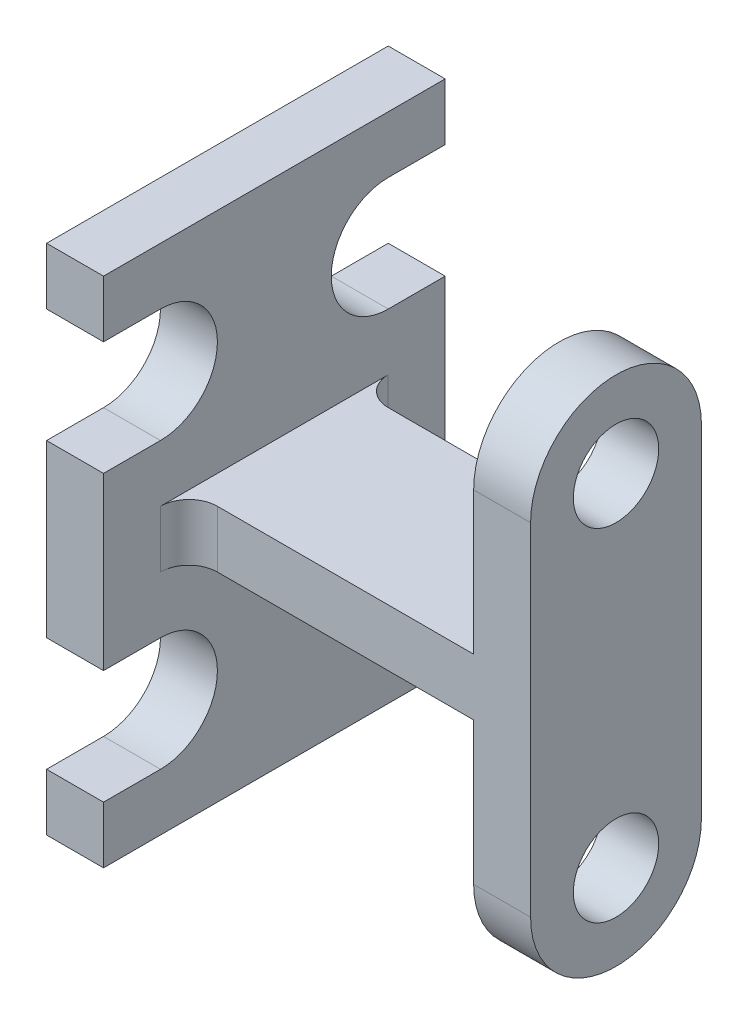
ISO-10303-21;
HEADER;
FILE_DESCRIPTION(('STEP AP214'),'2;1');
FILE_NAME('part.step','',(''),(''),'','','');
FILE_SCHEMA(('AUTOMOTIVE_DESIGN { 1 0 10303 214 1 1 1 1 }'));
ENDSEC;
DATA;
#1=APPLICATION_CONTEXT('core data for automotive mechanical design processes');
#2=APPLICATION_PROTOCOL_DEFINITION('international standard','automotive_design',2000,#1);
#3=PRODUCT_CONTEXT('',#1,'mechanical');
#4=PRODUCT('Part','Part','',(#3));
#5=PRODUCT_RELATED_PRODUCT_CATEGORY('part','',(#4));
#6=PRODUCT_DEFINITION_FORMATION('','',#4);
#7=PRODUCT_DEFINITION_CONTEXT('part definition',#1,'design');
#8=PRODUCT_DEFINITION('design','',#6,#7);
#9=PRODUCT_DEFINITION_SHAPE('','',#8);
#10=(LENGTH_UNIT() NAMED_UNIT(*) SI_UNIT(.MILLI.,.METRE.));
#11=(NAMED_UNIT(*) PLANE_ANGLE_UNIT() SI_UNIT($,.RADIAN.));
#12=(NAMED_UNIT(*) SI_UNIT($,.STERADIAN.) SOLID_ANGLE_UNIT());
#13=UNCERTAINTY_MEASURE_WITH_UNIT(LENGTH_MEASURE(1.E-05),#10,'distance_accuracy_value','');
#14=(GEOMETRIC_REPRESENTATION_CONTEXT(3) GLOBAL_UNCERTAINTY_ASSIGNED_CONTEXT((#13)) GLOBAL_UNIT_ASSIGNED_CONTEXT((#10,
#11,#12)) REPRESENTATION_CONTEXT('',''));
#15=CARTESIAN_POINT('',(0.,0.,0.));
#16=DIRECTION('',(0.,0.,1.));
#17=DIRECTION('',(1.,0.,0.));
#18=AXIS2_PLACEMENT_3D('',#15,#16,#17);
#19=CARTESIAN_POINT('',(10.,4.99999999999997,60.));
#20=DIRECTION('',(-1.,0.,0.));
#21=DIRECTION('',(0.,0.,1.));
#22=AXIS2_PLACEMENT_3D('',#19,#20,#21);
#23=PLANE('',#22);
#24=DIRECTION('',(0.,0.,-1.));
#25=VECTOR('',#24,1.);
#26=CARTESIAN_POINT('',(10.,4.99999999999997,60.));
#27=LINE('',#26,#25);
#28=CARTESIAN_POINT('',(10.,4.99999999999997,50.));
#29=VERTEX_POINT('',#28);
#30=CARTESIAN_POINT('',(10.,4.99999999999997,10.));
#31=VERTEX_POINT('',#30);
#32=EDGE_CURVE('E418',#29,#31,#27,.T.);
#33=ORIENTED_EDGE('',*,*,#32,.T.);
#34=DIRECTION('',(0.,1.,0.));
#35=VECTOR('',#34,1.);
#36=CARTESIAN_POINT('',(10.,-5.00000000000006,10.));
#37=LINE('',#36,#35);
#38=CARTESIAN_POINT('',(10.,-5.00000000000006,10.));
#39=VERTEX_POINT('',#38);
#40=EDGE_CURVE('E432',#31,#39,#37,.F.);
#41=ORIENTED_EDGE('',*,*,#40,.T.);
#42=DIRECTION('',(0.,0.,-1.));
#43=VECTOR('',#42,1.);
#44=CARTESIAN_POINT('',(10.,-5.00000000000006,60.));
#45=LINE('',#44,#43);
#46=CARTESIAN_POINT('',(10.,-5.00000000000006,50.));
#47=VERTEX_POINT('',#46);
#48=EDGE_CURVE('E423',#47,#39,#45,.T.);
#49=ORIENTED_EDGE('',*,*,#48,.F.);
#50=DIRECTION('',(0.,1.,0.));
#51=VECTOR('',#50,1.);
#52=CARTESIAN_POINT('',(10.,4.99999999999997,50.));
#53=LINE('',#52,#51);
#54=EDGE_CURVE('E431',#47,#29,#53,.T.);
#55=ORIENTED_EDGE('',*,*,#54,.T.);
#56=EDGE_LOOP('',(#33,#41,#49,#55));
#57=FACE_BOUND('',#56,.T.);
#58=DIRECTION('',(0.,1.,0.));
#59=VECTOR('',#58,1.);
#60=CARTESIAN_POINT('',(10.,4.99999999999997,60.));
#61=LINE('',#60,#59);
#62=CARTESIAN_POINT('',(10.,35.,60.));
#63=VERTEX_POINT('',#62);
#64=CARTESIAN_POINT('',(10.,45.,60.));
#65=VERTEX_POINT('',#64);
#66=EDGE_CURVE('E387',#63,#65,#61,.T.);
#67=ORIENTED_EDGE('',*,*,#66,.F.);
#68=DIRECTION('',(0.,0.,-1.));
#69=VECTOR('',#68,1.);
#70=CARTESIAN_POINT('',(10.,35.,0.));
#71=LINE('',#70,#69);
#72=CARTESIAN_POINT('',(10.,35.,50.));
#73=VERTEX_POINT('',#72);
#74=EDGE_CURVE('E311',#63,#73,#71,.T.);
#75=ORIENTED_EDGE('',*,*,#74,.T.);
#76=CARTESIAN_POINT('',(10.,25.,50.));
#77=DIRECTION('',(-1.,0.,0.));
#78=DIRECTION('',(0.,0.,1.));
#79=AXIS2_PLACEMENT_3D('',#76,#77,#78);
#80=CIRCLE('',#79,10.);
#81=CARTESIAN_POINT('',(10.,15.,50.));
#82=VERTEX_POINT('',#81);
#83=EDGE_CURVE('E304',#82,#73,#80,.F.);
#84=ORIENTED_EDGE('',*,*,#83,.F.);
#85=DIRECTION('',(0.,0.,1.));
#86=VECTOR('',#85,1.);
#87=CARTESIAN_POINT('',(10.,15.,0.));
#88=LINE('',#87,#86);
#89=CARTESIAN_POINT('',(10.,15.,60.));
#90=VERTEX_POINT('',#89);
#91=EDGE_CURVE('E310',#82,#90,#88,.T.);
#92=ORIENTED_EDGE('',*,*,#91,.T.);
#93=CARTESIAN_POINT('',(10.,-15.,60.));
#94=VERTEX_POINT('',#93);
#95=EDGE_CURVE('E394',#94,#90,#61,.T.);
#96=ORIENTED_EDGE('',*,*,#95,.F.);
#97=DIRECTION('',(0.,0.,-1.));
#98=VECTOR('',#97,1.);
#99=CARTESIAN_POINT('',(10.,-15.,0.));
#100=LINE('',#99,#98);
#101=CARTESIAN_POINT('',(10.,-15.,50.));
#102=VERTEX_POINT('',#101);
#103=EDGE_CURVE('E277',#94,#102,#100,.T.);
#104=ORIENTED_EDGE('',*,*,#103,.T.);
#105=CARTESIAN_POINT('',(10.,-24.9999999999999,50.));
#106=DIRECTION('',(-1.,0.,0.));
#107=DIRECTION('',(0.,0.,1.));
#108=AXIS2_PLACEMENT_3D('',#105,#106,#107);
#109=CIRCLE('',#108,9.99999999999998);
#110=CARTESIAN_POINT('',(10.,-34.9999999999999,50.));
#111=VERTEX_POINT('',#110);
#112=EDGE_CURVE('E285',#102,#111,#109,.T.);
#113=ORIENTED_EDGE('',*,*,#112,.T.);
#114=DIRECTION('',(0.,0.,1.));
#115=VECTOR('',#114,1.);
#116=CARTESIAN_POINT('',(10.,-35.,0.));
#117=LINE('',#116,#115);
#118=CARTESIAN_POINT('',(10.,-34.9999999999999,60.));
#119=VERTEX_POINT('',#118);
#120=EDGE_CURVE('E286',#111,#119,#117,.T.);
#121=ORIENTED_EDGE('',*,*,#120,.T.);
#122=DIRECTION('',(0.,1.,0.));
#123=VECTOR('',#122,1.);
#124=CARTESIAN_POINT('',(10.,-45.,60.));
#125=LINE('',#124,#123);
#126=CARTESIAN_POINT('',(10.,-45.,60.));
#127=VERTEX_POINT('',#126);
#128=EDGE_CURVE('E386',#127,#119,#125,.T.);
#129=ORIENTED_EDGE('',*,*,#128,.F.);
#130=DIRECTION('',(0.,0.,-1.));
#131=VECTOR('',#130,1.);
#132=CARTESIAN_POINT('',(10.,-45.,60.));
#133=LINE('',#132,#131);
#134=CARTESIAN_POINT('',(10.,-45.,0.));
#135=VERTEX_POINT('',#134);
#136=EDGE_CURVE('E421',#127,#135,#133,.T.);
#137=ORIENTED_EDGE('',*,*,#136,.T.);
#138=DIRECTION('',(0.,1.,0.));
#139=VECTOR('',#138,1.);
#140=CARTESIAN_POINT('',(10.,-45.,0.));
#141=LINE('',#140,#139);
#142=CARTESIAN_POINT('',(10.,-35.,0.));
#143=VERTEX_POINT('',#142);
#144=EDGE_CURVE('E399',#135,#143,#141,.T.);
#145=ORIENTED_EDGE('',*,*,#144,.T.);
#146=DIRECTION('',(0.,0.,-1.));
#147=VECTOR('',#146,1.);
#148=CARTESIAN_POINT('',(10.,-35.,0.));
#149=LINE('',#148,#147);
#150=CARTESIAN_POINT('',(10.,-35.,10.));
#151=VERTEX_POINT('',#150);
#152=EDGE_CURVE('E340',#151,#143,#149,.T.);
#153=ORIENTED_EDGE('',*,*,#152,.F.);
#154=CARTESIAN_POINT('',(10.,-25.,10.));
#155=DIRECTION('',(-1.,0.,0.));
#156=DIRECTION('',(0.,0.,1.));
#157=AXIS2_PLACEMENT_3D('',#154,#155,#156);
#158=CIRCLE('',#157,10.);
#159=CARTESIAN_POINT('',(10.,-15.,10.));
#160=VERTEX_POINT('',#159);
#161=EDGE_CURVE('E335',#160,#151,#158,.F.);
#162=ORIENTED_EDGE('',*,*,#161,.F.);
#163=DIRECTION('',(0.,0.,1.));
#164=VECTOR('',#163,1.);
#165=CARTESIAN_POINT('',(10.,-15.,0.));
#166=LINE('',#165,#164);
#167=CARTESIAN_POINT('',(10.,-15.,0.));
#168=VERTEX_POINT('',#167);
#169=EDGE_CURVE('E333',#168,#160,#166,.T.);
#170=ORIENTED_EDGE('',*,*,#169,.F.);
#171=DIRECTION('',(0.,1.,0.));
#172=VECTOR('',#171,1.);
#173=CARTESIAN_POINT('',(10.,4.99999999999997,0.));
#174=LINE('',#173,#172);
#175=CARTESIAN_POINT('',(10.,15.,0.));
#176=VERTEX_POINT('',#175);
#177=EDGE_CURVE('E404',#168,#176,#174,.T.);
#178=ORIENTED_EDGE('',*,*,#177,.T.);
#179=DIRECTION('',(0.,0.,-1.));
#180=VECTOR('',#179,1.);
#181=CARTESIAN_POINT('',(10.,15.,0.));
#182=LINE('',#181,#180);
#183=CARTESIAN_POINT('',(10.,15.,10.));
#184=VERTEX_POINT('',#183);
#185=EDGE_CURVE('E354',#184,#176,#182,.T.);
#186=ORIENTED_EDGE('',*,*,#185,.F.);
#187=CARTESIAN_POINT('',(10.,25.,10.));
#188=DIRECTION('',(-1.,0.,0.));
#189=DIRECTION('',(0.,0.,1.));
#190=AXIS2_PLACEMENT_3D('',#187,#188,#189);
#191=CIRCLE('',#190,10.);
#192=CARTESIAN_POINT('',(10.,35.,10.));
#193=VERTEX_POINT('',#192);
#194=EDGE_CURVE('E357',#184,#193,#191,.T.);
#195=ORIENTED_EDGE('',*,*,#194,.T.);
#196=DIRECTION('',(0.,0.,1.));
#197=VECTOR('',#196,1.);
#198=CARTESIAN_POINT('',(10.,35.,0.));
#199=LINE('',#198,#197);
#200=CARTESIAN_POINT('',(10.,35.,0.));
#201=VERTEX_POINT('',#200);
#202=EDGE_CURVE('E363',#201,#193,#199,.T.);
#203=ORIENTED_EDGE('',*,*,#202,.F.);
#204=CARTESIAN_POINT('',(10.,45.,0.));
#205=VERTEX_POINT('',#204);
#206=EDGE_CURVE('E401',#201,#205,#174,.T.);
#207=ORIENTED_EDGE('',*,*,#206,.T.);
#208=DIRECTION('',(0.,0.,-1.));
#209=VECTOR('',#208,1.);
#210=CARTESIAN_POINT('',(10.,45.,60.));
#211=LINE('',#210,#209);
#212=EDGE_CURVE('E416',#65,#205,#211,.T.);
#213=ORIENTED_EDGE('',*,*,#212,.F.);
#214=EDGE_LOOP('',(#67,#75,#84,#92,#96,#104,#113,#121,#129,#137,#145,#153,#162,#170,#178,#186,
#195,#203,#207,#213));
#215=FACE_BOUND('',#214,.T.);
#216=ADVANCED_FACE('F39',(#57,#215),#23,.F.);
#217=CARTESIAN_POINT('',(0.,0.,60.));
#218=DIRECTION('',(1.,0.,0.));
#219=DIRECTION('',(0.,0.,-1.));
#220=AXIS2_PLACEMENT_3D('',#217,#218,#219);
#221=PLANE('',#220);
#222=CARTESIAN_POINT('',(0.,25.,50.));
#223=DIRECTION('',(-1.,0.,0.));
#224=DIRECTION('',(0.,0.,1.));
#225=AXIS2_PLACEMENT_3D('',#222,#223,#224);
#226=CIRCLE('',#225,10.);
#227=CARTESIAN_POINT('',(0.,15.,50.));
#228=VERTEX_POINT('',#227);
#229=CARTESIAN_POINT('',(0.,35.,50.));
#230=VERTEX_POINT('',#229);
#231=EDGE_CURVE('E314',#228,#230,#226,.F.);
#232=ORIENTED_EDGE('',*,*,#231,.T.);
#233=DIRECTION('',(0.,0.,-1.));
#234=VECTOR('',#233,1.);
#235=CARTESIAN_POINT('',(0.,35.,0.));
#236=LINE('',#235,#234);
#237=CARTESIAN_POINT('',(0.,35.,60.));
#238=VERTEX_POINT('',#237);
#239=EDGE_CURVE('E308',#238,#230,#236,.T.);
#240=ORIENTED_EDGE('',*,*,#239,.F.);
#241=DIRECTION('',(0.,-1.,0.));
#242=VECTOR('',#241,1.);
#243=CARTESIAN_POINT('',(0.,0.,60.));
#244=LINE('',#243,#242);
#245=CARTESIAN_POINT('',(0.,45.,60.));
#246=VERTEX_POINT('',#245);
#247=EDGE_CURVE('E379',#246,#238,#244,.T.);
#248=ORIENTED_EDGE('',*,*,#247,.F.);
#249=DIRECTION('',(0.,0.,-1.));
#250=VECTOR('',#249,1.);
#251=CARTESIAN_POINT('',(0.,45.,60.));
#252=LINE('',#251,#250);
#253=CARTESIAN_POINT('',(0.,45.,0.));
#254=VERTEX_POINT('',#253);
#255=EDGE_CURVE('E400',#246,#254,#252,.T.);
#256=ORIENTED_EDGE('',*,*,#255,.T.);
#257=DIRECTION('',(0.,-1.,0.));
#258=VECTOR('',#257,1.);
#259=CARTESIAN_POINT('',(0.,0.,0.));
#260=LINE('',#259,#258);
#261=CARTESIAN_POINT('',(0.,35.,0.));
#262=VERTEX_POINT('',#261);
#263=EDGE_CURVE('E407',#254,#262,#260,.T.);
#264=ORIENTED_EDGE('',*,*,#263,.T.);
#265=DIRECTION('',(0.,0.,1.));
#266=VECTOR('',#265,1.);
#267=CARTESIAN_POINT('',(0.,35.,0.));
#268=LINE('',#267,#266);
#269=CARTESIAN_POINT('',(0.,35.,10.));
#270=VERTEX_POINT('',#269);
#271=EDGE_CURVE('E356',#262,#270,#268,.T.);
#272=ORIENTED_EDGE('',*,*,#271,.T.);
#273=CARTESIAN_POINT('',(0.,25.,10.));
#274=DIRECTION('',(-1.,0.,0.));
#275=DIRECTION('',(0.,0.,1.));
#276=AXIS2_PLACEMENT_3D('',#273,#274,#275);
#277=CIRCLE('',#276,10.);
#278=CARTESIAN_POINT('',(0.,15.,10.));
#279=VERTEX_POINT('',#278);
#280=EDGE_CURVE('E366',#279,#270,#277,.T.);
#281=ORIENTED_EDGE('',*,*,#280,.F.);
#282=DIRECTION('',(0.,0.,-1.));
#283=VECTOR('',#282,1.);
#284=CARTESIAN_POINT('',(0.,15.,0.));
#285=LINE('',#284,#283);
#286=CARTESIAN_POINT('',(0.,15.,0.));
#287=VERTEX_POINT('',#286);
#288=EDGE_CURVE('E322',#279,#287,#285,.T.);
#289=ORIENTED_EDGE('',*,*,#288,.T.);
#290=CARTESIAN_POINT('',(0.,-15.,0.));
#291=VERTEX_POINT('',#290);
#292=EDGE_CURVE('E415',#287,#291,#260,.T.);
#293=ORIENTED_EDGE('',*,*,#292,.T.);
#294=DIRECTION('',(0.,0.,1.));
#295=VECTOR('',#294,1.);
#296=CARTESIAN_POINT('',(0.,-15.,0.));
#297=LINE('',#296,#295);
#298=CARTESIAN_POINT('',(0.,-15.,10.));
#299=VERTEX_POINT('',#298);
#300=EDGE_CURVE('E341',#291,#299,#297,.T.);
#301=ORIENTED_EDGE('',*,*,#300,.T.);
#302=CARTESIAN_POINT('',(0.,-25.,10.));
#303=DIRECTION('',(-1.,0.,0.));
#304=DIRECTION('',(0.,0.,1.));
#305=AXIS2_PLACEMENT_3D('',#302,#303,#304);
#306=CIRCLE('',#305,10.);
#307=CARTESIAN_POINT('',(0.,-35.,10.));
#308=VERTEX_POINT('',#307);
#309=EDGE_CURVE('E296',#299,#308,#306,.F.);
#310=ORIENTED_EDGE('',*,*,#309,.T.);
#311=DIRECTION('',(0.,0.,-1.));
#312=VECTOR('',#311,1.);
#313=CARTESIAN_POINT('',(0.,-35.,0.));
#314=LINE('',#313,#312);
#315=CARTESIAN_POINT('',(0.,-35.,0.));
#316=VERTEX_POINT('',#315);
#317=EDGE_CURVE('E334',#308,#316,#314,.T.);
#318=ORIENTED_EDGE('',*,*,#317,.T.);
#319=CARTESIAN_POINT('',(0.,-45.,0.));
#320=VERTEX_POINT('',#319);
#321=EDGE_CURVE('E408',#316,#320,#260,.T.);
#322=ORIENTED_EDGE('',*,*,#321,.T.);
#323=DIRECTION('',(0.,0.,-1.));
#324=VECTOR('',#323,1.);
#325=CARTESIAN_POINT('',(0.,-45.,60.));
#326=LINE('',#325,#324);
#327=CARTESIAN_POINT('',(0.,-45.,60.));
#328=VERTEX_POINT('',#327);
#329=EDGE_CURVE('E424',#328,#320,#326,.T.);
#330=ORIENTED_EDGE('',*,*,#329,.F.);
#331=CARTESIAN_POINT('',(0.,-34.9999999999999,60.));
#332=VERTEX_POINT('',#331);
#333=EDGE_CURVE('E383',#332,#328,#244,.T.);
#334=ORIENTED_EDGE('',*,*,#333,.F.);
#335=DIRECTION('',(0.,0.,1.));
#336=VECTOR('',#335,1.);
#337=CARTESIAN_POINT('',(0.,-35.,0.));
#338=LINE('',#337,#336);
#339=CARTESIAN_POINT('',(0.,-34.9999999999999,50.));
#340=VERTEX_POINT('',#339);
#341=EDGE_CURVE('E283',#340,#332,#338,.T.);
#342=ORIENTED_EDGE('',*,*,#341,.F.);
#343=CARTESIAN_POINT('',(0.,-24.9999999999999,50.));
#344=DIRECTION('',(-1.,0.,0.));
#345=DIRECTION('',(0.,0.,1.));
#346=AXIS2_PLACEMENT_3D('',#343,#344,#345);
#347=CIRCLE('',#346,9.99999999999998);
#348=CARTESIAN_POINT('',(0.,-15.,50.));
#349=VERTEX_POINT('',#348);
#350=EDGE_CURVE('E292',#349,#340,#347,.T.);
#351=ORIENTED_EDGE('',*,*,#350,.F.);
#352=DIRECTION('',(0.,0.,-1.));
#353=VECTOR('',#352,1.);
#354=CARTESIAN_POINT('',(0.,-15.,0.));
#355=LINE('',#354,#353);
#356=CARTESIAN_POINT('',(0.,-15.,60.));
#357=VERTEX_POINT('',#356);
#358=EDGE_CURVE('E247',#357,#349,#355,.T.);
#359=ORIENTED_EDGE('',*,*,#358,.F.);
#360=CARTESIAN_POINT('',(0.,15.,60.));
#361=VERTEX_POINT('',#360);
#362=EDGE_CURVE('E381',#361,#357,#244,.T.);
#363=ORIENTED_EDGE('',*,*,#362,.F.);
#364=DIRECTION('',(0.,0.,1.));
#365=VECTOR('',#364,1.);
#366=CARTESIAN_POINT('',(0.,15.,0.));
#367=LINE('',#366,#365);
#368=EDGE_CURVE('E319',#228,#361,#367,.T.);
#369=ORIENTED_EDGE('',*,*,#368,.F.);
#370=EDGE_LOOP('',(#232,#240,#248,#256,#264,#272,#281,#289,#293,#301,#310,#318,#322,#330,#334,
#342,#351,#359,#363,#369));
#371=FACE_BOUND('',#370,.T.);
#372=ADVANCED_FACE('F499',(#371),#221,.F.);
#373=CARTESIAN_POINT('',(0.,0.,60.));
#374=DIRECTION('',(0.,0.,1.));
#375=DIRECTION('',(1.,0.,0.));
#376=AXIS2_PLACEMENT_3D('',#373,#374,#375);
#377=PLANE('',#376);
#378=DIRECTION('',(-1.,0.,0.));
#379=VECTOR('',#378,1.);
#380=CARTESIAN_POINT('',(10.,35.,60.));
#381=LINE('',#380,#379);
#382=EDGE_CURVE('E329',#63,#238,#381,.T.);
#383=ORIENTED_EDGE('',*,*,#382,.F.);
#384=ORIENTED_EDGE('',*,*,#66,.T.);
#385=DIRECTION('',(-1.,0.,0.));
#386=VECTOR('',#385,1.);
#387=CARTESIAN_POINT('',(10.,45.,60.));
#388=LINE('',#387,#386);
#389=EDGE_CURVE('E393',#65,#246,#388,.T.);
#390=ORIENTED_EDGE('',*,*,#389,.T.);
#391=ORIENTED_EDGE('',*,*,#247,.T.);
#392=EDGE_LOOP('',(#383,#384,#390,#391));
#393=FACE_BOUND('',#392,.T.);
#394=ADVANCED_FACE('F507',(#393),#377,.T.);
#395=DIRECTION('',(-1.,0.,0.));
#396=VECTOR('',#395,1.);
#397=CARTESIAN_POINT('',(10.,-15.,60.));
#398=LINE('',#397,#396);
#399=EDGE_CURVE('E298',#94,#357,#398,.T.);
#400=ORIENTED_EDGE('',*,*,#399,.F.);
#401=ORIENTED_EDGE('',*,*,#95,.T.);
#402=DIRECTION('',(-1.,0.,0.));
#403=VECTOR('',#402,1.);
#404=CARTESIAN_POINT('',(10.,15.,60.));
#405=LINE('',#404,#403);
#406=EDGE_CURVE('E330',#90,#361,#405,.T.);
#407=ORIENTED_EDGE('',*,*,#406,.T.);
#408=ORIENTED_EDGE('',*,*,#362,.T.);
#409=EDGE_LOOP('',(#400,#401,#407,#408));
#410=FACE_BOUND('',#409,.T.);
#411=ADVANCED_FACE('F747',(#410),#377,.T.);
#412=CARTESIAN_POINT('',(0.,0.,0.));
#413=DIRECTION('',(0.,0.,1.));
#414=DIRECTION('',(1.,0.,0.));
#415=AXIS2_PLACEMENT_3D('',#412,#413,#414);
#416=PLANE('',#415);
#417=DIRECTION('',(-1.,0.,0.));
#418=VECTOR('',#417,1.);
#419=CARTESIAN_POINT('',(10.,-35.,0.));
#420=LINE('',#419,#418);
#421=EDGE_CURVE('E348',#143,#316,#420,.T.);
#422=ORIENTED_EDGE('',*,*,#421,.F.);
#423=ORIENTED_EDGE('',*,*,#144,.F.);
#424=DIRECTION('',(1.,0.,0.));
#425=VECTOR('',#424,1.);
#426=CARTESIAN_POINT('',(0.,-45.,0.));
#427=LINE('',#426,#425);
#428=EDGE_CURVE('E373',#320,#135,#427,.T.);
#429=ORIENTED_EDGE('',*,*,#428,.F.);
#430=ORIENTED_EDGE('',*,*,#321,.F.);
#431=EDGE_LOOP('',(#422,#423,#429,#430));
#432=FACE_BOUND('',#431,.T.);
#433=ADVANCED_FACE('F757',(#432),#416,.F.);
#434=ORIENTED_EDGE('',*,*,#177,.F.);
#435=DIRECTION('',(-1.,0.,0.));
#436=VECTOR('',#435,1.);
#437=CARTESIAN_POINT('',(10.,-15.,0.));
#438=LINE('',#437,#436);
#439=EDGE_CURVE('E351',#168,#291,#438,.T.);
#440=ORIENTED_EDGE('',*,*,#439,.T.);
#441=ORIENTED_EDGE('',*,*,#292,.F.);
#442=DIRECTION('',(-1.,0.,0.));
#443=VECTOR('',#442,1.);
#444=CARTESIAN_POINT('',(10.,15.,0.));
#445=LINE('',#444,#443);
#446=EDGE_CURVE('E371',#176,#287,#445,.T.);
#447=ORIENTED_EDGE('',*,*,#446,.F.);
#448=EDGE_LOOP('',(#434,#440,#441,#447));
#449=FACE_BOUND('',#448,.T.);
#450=ADVANCED_FACE('F756',(#449),#416,.F.);
#451=DIRECTION('',(-1.,0.,0.));
#452=VECTOR('',#451,1.);
#453=CARTESIAN_POINT('',(10.,35.,0.));
#454=LINE('',#453,#452);
#455=EDGE_CURVE('E372',#201,#262,#454,.T.);
#456=ORIENTED_EDGE('',*,*,#455,.T.);
#457=ORIENTED_EDGE('',*,*,#263,.F.);
#458=DIRECTION('',(-1.,0.,0.));
#459=VECTOR('',#458,1.);
#460=CARTESIAN_POINT('',(10.,45.,0.));
#461=LINE('',#460,#459);
#462=EDGE_CURVE('E406',#205,#254,#461,.T.);
#463=ORIENTED_EDGE('',*,*,#462,.F.);
#464=ORIENTED_EDGE('',*,*,#206,.F.);
#465=EDGE_LOOP('',(#456,#457,#463,#464));
#466=FACE_BOUND('',#465,.T.);
#467=ADVANCED_FACE('F517',(#466),#416,.F.);
#468=CARTESIAN_POINT('',(0.,-45.,60.));
#469=DIRECTION('',(0.,1.,0.));
#470=DIRECTION('',(0.,0.,1.));
#471=AXIS2_PLACEMENT_3D('',#468,#469,#470);
#472=PLANE('',#471);
#473=ORIENTED_EDGE('',*,*,#428,.T.);
#474=ORIENTED_EDGE('',*,*,#136,.F.);
#475=DIRECTION('',(1.,0.,0.));
#476=VECTOR('',#475,1.);
#477=CARTESIAN_POINT('',(0.,-45.,60.));
#478=LINE('',#477,#476);
#479=EDGE_CURVE('E384',#328,#127,#478,.T.);
#480=ORIENTED_EDGE('',*,*,#479,.F.);
#481=ORIENTED_EDGE('',*,*,#329,.T.);
#482=EDGE_LOOP('',(#473,#474,#480,#481));
#483=FACE_BOUND('',#482,.T.);
#484=ADVANCED_FACE('F520',(#483),#472,.F.);
#485=CARTESIAN_POINT('',(50.,-5.00000000000005,60.));
#486=DIRECTION('',(0.,1.,0.));
#487=DIRECTION('',(-1.,0.,0.));
#488=AXIS2_PLACEMENT_3D('',#485,#486,#487);
#489=PLANE('',#488);
#490=ORIENTED_EDGE('',*,*,#48,.T.);
#491=CARTESIAN_POINT('',(15.,-5.00000000000006,10.));
#492=DIRECTION('',(0.,1.,0.));
#493=DIRECTION('',(-1.,0.,0.));
#494=AXIS2_PLACEMENT_3D('',#491,#492,#493);
#495=CIRCLE('',#494,5.);
#496=CARTESIAN_POINT('',(15.,-5.00000000000006,15.));
#497=VERTEX_POINT('',#496);
#498=EDGE_CURVE('E441',#39,#497,#495,.T.);
#499=ORIENTED_EDGE('',*,*,#498,.T.);
#500=DIRECTION('',(1.,0.,0.));
#501=VECTOR('',#500,1.);
#502=CARTESIAN_POINT('',(50.,-5.00000000000005,15.));
#503=LINE('',#502,#501);
#504=CARTESIAN_POINT('',(60.,-5.00000000000006,15.));
#505=VERTEX_POINT('',#504);
#506=EDGE_CURVE('E450',#497,#505,#503,.T.);
#507=ORIENTED_EDGE('',*,*,#506,.T.);
#508=DIRECTION('',(0.,0.,-1.));
#509=VECTOR('',#508,1.);
#510=CARTESIAN_POINT('',(60.,-5.00000000000005,0.));
#511=LINE('',#510,#509);
#512=CARTESIAN_POINT('',(60.,-5.00000000000005,45.));
#513=VERTEX_POINT('',#512);
#514=EDGE_CURVE('E248',#513,#505,#511,.T.);
#515=ORIENTED_EDGE('',*,*,#514,.F.);
#516=DIRECTION('',(-1.,0.,0.));
#517=VECTOR('',#516,1.);
#518=CARTESIAN_POINT('',(50.,-5.00000000000005,45.));
#519=LINE('',#518,#517);
#520=CARTESIAN_POINT('',(15.,-5.00000000000006,45.));
#521=VERTEX_POINT('',#520);
#522=EDGE_CURVE('E452',#513,#521,#519,.T.);
#523=ORIENTED_EDGE('',*,*,#522,.T.);
#524=CARTESIAN_POINT('',(15.,-5.00000000000006,50.));
#525=DIRECTION('',(0.,1.,0.));
#526=DIRECTION('',(-1.,0.,0.));
#527=AXIS2_PLACEMENT_3D('',#524,#525,#526);
#528=CIRCLE('',#527,5.);
#529=EDGE_CURVE('E11',#521,#47,#528,.T.);
#530=ORIENTED_EDGE('',*,*,#529,.T.);
#531=EDGE_LOOP('',(#490,#499,#507,#515,#523,#530));
#532=FACE_BOUND('',#531,.T.);
#533=ADVANCED_FACE('F444',(#532),#489,.F.);
#534=CARTESIAN_POINT('',(10.,4.99999999999997,60.));
#535=DIRECTION('',(0.,-1.,0.));
#536=DIRECTION('',(1.,0.,0.));
#537=AXIS2_PLACEMENT_3D('',#534,#535,#536);
#538=PLANE('',#537);
#539=DIRECTION('',(0.,0.,1.));
#540=VECTOR('',#539,1.);
#541=CARTESIAN_POINT('',(60.,4.99999999999997,0.));
#542=LINE('',#541,#540);
#543=CARTESIAN_POINT('',(60.,4.99999999999997,15.));
#544=VERTEX_POINT('',#543);
#545=CARTESIAN_POINT('',(60.,4.99999999999996,45.));
#546=VERTEX_POINT('',#545);
#547=EDGE_CURVE('E240',#544,#546,#542,.T.);
#548=ORIENTED_EDGE('',*,*,#547,.F.);
#549=DIRECTION('',(1.,0.,0.));
#550=VECTOR('',#549,1.);
#551=CARTESIAN_POINT('',(60.,4.99999999999996,15.));
#552=LINE('',#551,#550);
#553=CARTESIAN_POINT('',(15.,4.99999999999997,15.));
#554=VERTEX_POINT('',#553);
#555=EDGE_CURVE('E239',#554,#544,#552,.T.);
#556=ORIENTED_EDGE('',*,*,#555,.F.);
#557=CARTESIAN_POINT('',(15.,4.99999999999997,10.));
#558=DIRECTION('',(0.,-1.,0.));
#559=DIRECTION('',(1.,0.,0.));
#560=AXIS2_PLACEMENT_3D('',#557,#558,#559);
#561=CIRCLE('',#560,5.);
#562=EDGE_CURVE('E438',#554,#31,#561,.T.);
#563=ORIENTED_EDGE('',*,*,#562,.T.);
#564=ORIENTED_EDGE('',*,*,#32,.F.);
#565=CARTESIAN_POINT('',(15.,4.99999999999997,50.));
#566=DIRECTION('',(0.,-1.,0.));
#567=DIRECTION('',(1.,0.,0.));
#568=AXIS2_PLACEMENT_3D('',#565,#566,#567);
#569=CIRCLE('',#568,5.);
#570=CARTESIAN_POINT('',(15.,4.99999999999997,45.));
#571=VERTEX_POINT('',#570);
#572=EDGE_CURVE('E50',#29,#571,#569,.T.);
#573=ORIENTED_EDGE('',*,*,#572,.T.);
#574=DIRECTION('',(-1.,0.,0.));
#575=VECTOR('',#574,1.);
#576=CARTESIAN_POINT('',(60.,4.99999999999996,45.));
#577=LINE('',#576,#575);
#578=EDGE_CURVE('E231',#546,#571,#577,.T.);
#579=ORIENTED_EDGE('',*,*,#578,.F.);
#580=EDGE_LOOP('',(#548,#556,#563,#564,#573,#579));
#581=FACE_BOUND('',#580,.T.);
#582=ADVANCED_FACE('F232',(#581),#538,.F.);
#583=CARTESIAN_POINT('',(10.,45.,60.));
#584=DIRECTION('',(0.,-1.,0.));
#585=DIRECTION('',(0.,0.,-1.));
#586=AXIS2_PLACEMENT_3D('',#583,#584,#585);
#587=PLANE('',#586);
#588=ORIENTED_EDGE('',*,*,#462,.T.);
#589=ORIENTED_EDGE('',*,*,#255,.F.);
#590=ORIENTED_EDGE('',*,*,#389,.F.);
#591=ORIENTED_EDGE('',*,*,#212,.T.);
#592=EDGE_LOOP('',(#588,#589,#590,#591));
#593=FACE_BOUND('',#592,.T.);
#594=ADVANCED_FACE('F511',(#593),#587,.F.);
#595=DIRECTION('',(-1.,0.,0.));
#596=VECTOR('',#595,1.);
#597=CARTESIAN_POINT('',(10.,-34.9999999999999,60.));
#598=LINE('',#597,#596);
#599=EDGE_CURVE('E299',#119,#332,#598,.T.);
#600=ORIENTED_EDGE('',*,*,#599,.T.);
#601=ORIENTED_EDGE('',*,*,#333,.T.);
#602=ORIENTED_EDGE('',*,*,#479,.T.);
#603=ORIENTED_EDGE('',*,*,#128,.T.);
#604=EDGE_LOOP('',(#600,#601,#602,#603));
#605=FACE_BOUND('',#604,.T.);
#606=ADVANCED_FACE('F736',(#605),#377,.T.);
#607=CARTESIAN_POINT('',(10.,15.,0.));
#608=DIRECTION('',(0.,1.,0.));
#609=DIRECTION('',(0.,0.,1.));
#610=AXIS2_PLACEMENT_3D('',#607,#608,#609);
#611=PLANE('',#610);
#612=ORIENTED_EDGE('',*,*,#288,.F.);
#613=DIRECTION('',(-1.,0.,0.));
#614=VECTOR('',#613,1.);
#615=CARTESIAN_POINT('',(10.,15.,10.));
#616=LINE('',#615,#614);
#617=EDGE_CURVE('E361',#184,#279,#616,.T.);
#618=ORIENTED_EDGE('',*,*,#617,.F.);
#619=ORIENTED_EDGE('',*,*,#185,.T.);
#620=ORIENTED_EDGE('',*,*,#446,.T.);
#621=EDGE_LOOP('',(#612,#618,#619,#620));
#622=FACE_BOUND('',#621,.T.);
#623=ADVANCED_FACE('F726',(#622),#611,.T.);
#624=CARTESIAN_POINT('',(10.,35.,0.));
#625=DIRECTION('',(0.,-1.,0.));
#626=DIRECTION('',(0.,0.,-1.));
#627=AXIS2_PLACEMENT_3D('',#624,#625,#626);
#628=PLANE('',#627);
#629=ORIENTED_EDGE('',*,*,#271,.F.);
#630=ORIENTED_EDGE('',*,*,#455,.F.);
#631=ORIENTED_EDGE('',*,*,#202,.T.);
#632=DIRECTION('',(-1.,0.,0.));
#633=VECTOR('',#632,1.);
#634=CARTESIAN_POINT('',(10.,35.,10.));
#635=LINE('',#634,#633);
#636=EDGE_CURVE('E380',#193,#270,#635,.T.);
#637=ORIENTED_EDGE('',*,*,#636,.T.);
#638=EDGE_LOOP('',(#629,#630,#631,#637));
#639=FACE_BOUND('',#638,.T.);
#640=ADVANCED_FACE('F718',(#639),#628,.T.);
#641=CARTESIAN_POINT('',(10.,25.,10.));
#642=DIRECTION('',(-1.,0.,0.));
#643=DIRECTION('',(0.,0.,1.));
#644=AXIS2_PLACEMENT_3D('',#641,#642,#643);
#645=CYLINDRICAL_SURFACE('',#644,10.);
#646=ORIENTED_EDGE('',*,*,#280,.T.);
#647=ORIENTED_EDGE('',*,*,#636,.F.);
#648=ORIENTED_EDGE('',*,*,#194,.F.);
#649=ORIENTED_EDGE('',*,*,#617,.T.);
#650=EDGE_LOOP('',(#646,#647,#648,#649));
#651=FACE_BOUND('',#650,.T.);
#652=ADVANCED_FACE('F712',(#651),#645,.F.);
#653=CARTESIAN_POINT('',(10.,-25.,10.));
#654=DIRECTION('',(-1.,0.,0.));
#655=DIRECTION('',(0.,0.,1.));
#656=AXIS2_PLACEMENT_3D('',#653,#654,#655);
#657=CYLINDRICAL_SURFACE('',#656,10.);
#658=ORIENTED_EDGE('',*,*,#309,.F.);
#659=DIRECTION('',(-1.,0.,0.));
#660=VECTOR('',#659,1.);
#661=CARTESIAN_POINT('',(10.,-15.,10.));
#662=LINE('',#661,#660);
#663=EDGE_CURVE('E339',#160,#299,#662,.T.);
#664=ORIENTED_EDGE('',*,*,#663,.F.);
#665=ORIENTED_EDGE('',*,*,#161,.T.);
#666=DIRECTION('',(-1.,0.,0.));
#667=VECTOR('',#666,1.);
#668=CARTESIAN_POINT('',(10.,-35.,10.));
#669=LINE('',#668,#667);
#670=EDGE_CURVE('E316',#151,#308,#669,.T.);
#671=ORIENTED_EDGE('',*,*,#670,.T.);
#672=EDGE_LOOP('',(#658,#664,#665,#671));
#673=FACE_BOUND('',#672,.T.);
#674=ADVANCED_FACE('F709',(#673),#657,.F.);
#675=CARTESIAN_POINT('',(10.,-35.,0.));
#676=DIRECTION('',(0.,1.,0.));
#677=DIRECTION('',(0.,0.,1.));
#678=AXIS2_PLACEMENT_3D('',#675,#676,#677);
#679=PLANE('',#678);
#680=ORIENTED_EDGE('',*,*,#317,.F.);
#681=ORIENTED_EDGE('',*,*,#670,.F.);
#682=ORIENTED_EDGE('',*,*,#152,.T.);
#683=ORIENTED_EDGE('',*,*,#421,.T.);
#684=EDGE_LOOP('',(#680,#681,#682,#683));
#685=FACE_BOUND('',#684,.T.);
#686=ADVANCED_FACE('F697',(#685),#679,.T.);
#687=CARTESIAN_POINT('',(10.,-15.,0.));
#688=DIRECTION('',(0.,-1.,0.));
#689=DIRECTION('',(0.,0.,-1.));
#690=AXIS2_PLACEMENT_3D('',#687,#688,#689);
#691=PLANE('',#690);
#692=ORIENTED_EDGE('',*,*,#300,.F.);
#693=ORIENTED_EDGE('',*,*,#439,.F.);
#694=ORIENTED_EDGE('',*,*,#169,.T.);
#695=ORIENTED_EDGE('',*,*,#663,.T.);
#696=EDGE_LOOP('',(#692,#693,#694,#695));
#697=FACE_BOUND('',#696,.T.);
#698=ADVANCED_FACE('F687',(#697),#691,.T.);
#699=CARTESIAN_POINT('',(10.,-15.,0.));
#700=DIRECTION('',(0.,1.,0.));
#701=DIRECTION('',(0.,0.,1.));
#702=AXIS2_PLACEMENT_3D('',#699,#700,#701);
#703=PLANE('',#702);
#704=ORIENTED_EDGE('',*,*,#358,.T.);
#705=DIRECTION('',(-1.,0.,0.));
#706=VECTOR('',#705,1.);
#707=CARTESIAN_POINT('',(10.,-15.,50.));
#708=LINE('',#707,#706);
#709=EDGE_CURVE('E288',#102,#349,#708,.T.);
#710=ORIENTED_EDGE('',*,*,#709,.F.);
#711=ORIENTED_EDGE('',*,*,#103,.F.);
#712=ORIENTED_EDGE('',*,*,#399,.T.);
#713=EDGE_LOOP('',(#704,#710,#711,#712));
#714=FACE_BOUND('',#713,.T.);
#715=ADVANCED_FACE('F682',(#714),#703,.F.);
#716=CARTESIAN_POINT('',(10.,-35.,0.));
#717=DIRECTION('',(0.,-1.,0.));
#718=DIRECTION('',(0.,0.,-1.));
#719=AXIS2_PLACEMENT_3D('',#716,#717,#718);
#720=PLANE('',#719);
#721=ORIENTED_EDGE('',*,*,#341,.T.);
#722=ORIENTED_EDGE('',*,*,#599,.F.);
#723=ORIENTED_EDGE('',*,*,#120,.F.);
#724=DIRECTION('',(-1.,0.,0.));
#725=VECTOR('',#724,1.);
#726=CARTESIAN_POINT('',(10.,-34.9999999999999,50.));
#727=LINE('',#726,#725);
#728=EDGE_CURVE('E305',#111,#340,#727,.T.);
#729=ORIENTED_EDGE('',*,*,#728,.T.);
#730=EDGE_LOOP('',(#721,#722,#723,#729));
#731=FACE_BOUND('',#730,.T.);
#732=ADVANCED_FACE('F677',(#731),#720,.F.);
#733=CARTESIAN_POINT('',(10.,-24.9999999999999,50.));
#734=DIRECTION('',(-1.,0.,0.));
#735=DIRECTION('',(0.,0.,1.));
#736=AXIS2_PLACEMENT_3D('',#733,#734,#735);
#737=CYLINDRICAL_SURFACE('',#736,9.99999999999998);
#738=ORIENTED_EDGE('',*,*,#350,.T.);
#739=ORIENTED_EDGE('',*,*,#728,.F.);
#740=ORIENTED_EDGE('',*,*,#112,.F.);
#741=ORIENTED_EDGE('',*,*,#709,.T.);
#742=EDGE_LOOP('',(#738,#739,#740,#741));
#743=FACE_BOUND('',#742,.T.);
#744=ADVANCED_FACE('F674',(#743),#737,.F.);
#745=CARTESIAN_POINT('',(10.,25.,50.));
#746=DIRECTION('',(-1.,0.,0.));
#747=DIRECTION('',(0.,0.,1.));
#748=AXIS2_PLACEMENT_3D('',#745,#746,#747);
#749=CYLINDRICAL_SURFACE('',#748,10.);
#750=ORIENTED_EDGE('',*,*,#231,.F.);
#751=DIRECTION('',(-1.,0.,0.));
#752=VECTOR('',#751,1.);
#753=CARTESIAN_POINT('',(10.,15.,50.));
#754=LINE('',#753,#752);
#755=EDGE_CURVE('E313',#82,#228,#754,.T.);
#756=ORIENTED_EDGE('',*,*,#755,.F.);
#757=ORIENTED_EDGE('',*,*,#83,.T.);
#758=DIRECTION('',(-1.,0.,0.));
#759=VECTOR('',#758,1.);
#760=CARTESIAN_POINT('',(10.,35.,50.));
#761=LINE('',#760,#759);
#762=EDGE_CURVE('E325',#73,#230,#761,.T.);
#763=ORIENTED_EDGE('',*,*,#762,.T.);
#764=EDGE_LOOP('',(#750,#756,#757,#763));
#765=FACE_BOUND('',#764,.T.);
#766=ADVANCED_FACE('F665',(#765),#749,.F.);
#767=CARTESIAN_POINT('',(10.,35.,0.));
#768=DIRECTION('',(0.,1.,0.));
#769=DIRECTION('',(0.,0.,1.));
#770=AXIS2_PLACEMENT_3D('',#767,#768,#769);
#771=PLANE('',#770);
#772=ORIENTED_EDGE('',*,*,#239,.T.);
#773=ORIENTED_EDGE('',*,*,#762,.F.);
#774=ORIENTED_EDGE('',*,*,#74,.F.);
#775=ORIENTED_EDGE('',*,*,#382,.T.);
#776=EDGE_LOOP('',(#772,#773,#774,#775));
#777=FACE_BOUND('',#776,.T.);
#778=ADVANCED_FACE('F653',(#777),#771,.F.);
#779=CARTESIAN_POINT('',(10.,15.,0.));
#780=DIRECTION('',(0.,-1.,0.));
#781=DIRECTION('',(0.,0.,-1.));
#782=AXIS2_PLACEMENT_3D('',#779,#780,#781);
#783=PLANE('',#782);
#784=ORIENTED_EDGE('',*,*,#368,.T.);
#785=ORIENTED_EDGE('',*,*,#406,.F.);
#786=ORIENTED_EDGE('',*,*,#91,.F.);
#787=ORIENTED_EDGE('',*,*,#755,.T.);
#788=EDGE_LOOP('',(#784,#785,#786,#787));
#789=FACE_BOUND('',#788,.T.);
#790=ADVANCED_FACE('F543',(#789),#783,.F.);
#791=CARTESIAN_POINT('',(60.,30.,30.));
#792=DIRECTION('',(1.,0.,0.));
#793=DIRECTION('',(0.,0.,-1.));
#794=AXIS2_PLACEMENT_3D('',#791,#792,#793);
#795=PLANE('',#794);
#796=CARTESIAN_POINT('',(60.,-30.,30.));
#797=DIRECTION('',(1.,0.,0.));
#798=DIRECTION('',(0.,0.,-1.));
#799=AXIS2_PLACEMENT_3D('',#796,#797,#798);
#800=CIRCLE('',#799,7.5);
#801=CARTESIAN_POINT('',(60.,-30.,22.5));
#802=VERTEX_POINT('',#801);
#803=EDGE_CURVE('E453',#802,#802,#800,.T.);
#804=ORIENTED_EDGE('',*,*,#803,.T.);
#805=EDGE_LOOP('',(#804));
#806=FACE_BOUND('',#805,.T.);
#807=DIRECTION('',(0.,-1.,0.));
#808=VECTOR('',#807,1.);
#809=CARTESIAN_POINT('',(60.,30.,45.));
#810=LINE('',#809,#808);
#811=CARTESIAN_POINT('',(60.,-30.,45.));
#812=VERTEX_POINT('',#811);
#813=EDGE_CURVE('E259',#513,#812,#810,.T.);
#814=ORIENTED_EDGE('',*,*,#813,.F.);
#815=ORIENTED_EDGE('',*,*,#514,.T.);
#816=DIRECTION('',(0.,1.,0.));
#817=VECTOR('',#816,1.);
#818=CARTESIAN_POINT('',(60.,30.,15.));
#819=LINE('',#818,#817);
#820=CARTESIAN_POINT('',(60.,-30.,15.));
#821=VERTEX_POINT('',#820);
#822=EDGE_CURVE('E265',#821,#505,#819,.T.);
#823=ORIENTED_EDGE('',*,*,#822,.F.);
#824=CARTESIAN_POINT('',(60.,-30.,30.));
#825=DIRECTION('',(1.,0.,0.));
#826=DIRECTION('',(0.,0.,-1.));
#827=AXIS2_PLACEMENT_3D('',#824,#825,#826);
#828=CIRCLE('',#827,15.);
#829=EDGE_CURVE('E253',#812,#821,#828,.T.);
#830=ORIENTED_EDGE('',*,*,#829,.F.);
#831=EDGE_LOOP('',(#814,#815,#823,#830));
#832=FACE_BOUND('',#831,.T.);
#833=ADVANCED_FACE('F544',(#806,#832),#795,.F.);
#834=CARTESIAN_POINT('',(60.,30.,30.));
#835=DIRECTION('',(1.,0.,0.));
#836=DIRECTION('',(0.,0.,-1.));
#837=AXIS2_PLACEMENT_3D('',#834,#835,#836);
#838=CIRCLE('',#837,7.5);
#839=CARTESIAN_POINT('',(60.,30.,22.5));
#840=VERTEX_POINT('',#839);
#841=EDGE_CURVE('E463',#840,#840,#838,.T.);
#842=ORIENTED_EDGE('',*,*,#841,.T.);
#843=EDGE_LOOP('',(#842));
#844=FACE_BOUND('',#843,.T.);
#845=CARTESIAN_POINT('',(60.,30.,15.));
#846=VERTEX_POINT('',#845);
#847=EDGE_CURVE('E250',#544,#846,#819,.T.);
#848=ORIENTED_EDGE('',*,*,#847,.F.);
#849=ORIENTED_EDGE('',*,*,#547,.T.);
#850=CARTESIAN_POINT('',(60.,30.,45.));
#851=VERTEX_POINT('',#850);
#852=EDGE_CURVE('E244',#851,#546,#810,.T.);
#853=ORIENTED_EDGE('',*,*,#852,.F.);
#854=CARTESIAN_POINT('',(60.,30.,30.));
#855=DIRECTION('',(1.,0.,0.));
#856=DIRECTION('',(0.,0.,-1.));
#857=AXIS2_PLACEMENT_3D('',#854,#855,#856);
#858=CIRCLE('',#857,15.);
#859=EDGE_CURVE('E258',#846,#851,#858,.T.);
#860=ORIENTED_EDGE('',*,*,#859,.F.);
#861=EDGE_LOOP('',(#848,#849,#853,#860));
#862=FACE_BOUND('',#861,.T.);
#863=ADVANCED_FACE('F243',(#844,#862),#795,.F.);
#864=CARTESIAN_POINT('',(70.,30.,30.));
#865=DIRECTION('',(1.,0.,0.));
#866=DIRECTION('',(0.,0.,-1.));
#867=AXIS2_PLACEMENT_3D('',#864,#865,#866);
#868=PLANE('',#867);
#869=CARTESIAN_POINT('',(70.,30.,30.));
#870=DIRECTION('',(1.,0.,0.));
#871=DIRECTION('',(0.,0.,-1.));
#872=AXIS2_PLACEMENT_3D('',#869,#870,#871);
#873=CIRCLE('',#872,7.5);
#874=CARTESIAN_POINT('',(70.,30.,22.5));
#875=VERTEX_POINT('',#874);
#876=EDGE_CURVE('E470',#875,#875,#873,.T.);
#877=ORIENTED_EDGE('',*,*,#876,.F.);
#878=EDGE_LOOP('',(#877));
#879=FACE_BOUND('',#878,.T.);
#880=CARTESIAN_POINT('',(70.,30.,30.));
#881=DIRECTION('',(1.,0.,0.));
#882=DIRECTION('',(0.,0.,-1.));
#883=AXIS2_PLACEMENT_3D('',#880,#881,#882);
#884=CIRCLE('',#883,15.);
#885=CARTESIAN_POINT('',(70.,30.,15.));
#886=VERTEX_POINT('',#885);
#887=CARTESIAN_POINT('',(70.,30.,45.));
#888=VERTEX_POINT('',#887);
#889=EDGE_CURVE('E266',#886,#888,#884,.T.);
#890=ORIENTED_EDGE('',*,*,#889,.T.);
#891=DIRECTION('',(0.,-1.,0.));
#892=VECTOR('',#891,1.);
#893=CARTESIAN_POINT('',(70.,30.,45.));
#894=LINE('',#893,#892);
#895=CARTESIAN_POINT('',(70.,-30.,45.));
#896=VERTEX_POINT('',#895);
#897=EDGE_CURVE('E473',#888,#896,#894,.T.);
#898=ORIENTED_EDGE('',*,*,#897,.T.);
#899=CARTESIAN_POINT('',(70.,-30.,30.));
#900=DIRECTION('',(1.,0.,0.));
#901=DIRECTION('',(0.,0.,-1.));
#902=AXIS2_PLACEMENT_3D('',#899,#900,#901);
#903=CIRCLE('',#902,15.);
#904=CARTESIAN_POINT('',(70.,-30.,15.));
#905=VERTEX_POINT('',#904);
#906=EDGE_CURVE('E479',#896,#905,#903,.T.);
#907=ORIENTED_EDGE('',*,*,#906,.T.);
#908=DIRECTION('',(0.,1.,0.));
#909=VECTOR('',#908,1.);
#910=CARTESIAN_POINT('',(70.,30.,15.));
#911=LINE('',#910,#909);
#912=EDGE_CURVE('E272',#905,#886,#911,.T.);
#913=ORIENTED_EDGE('',*,*,#912,.T.);
#914=EDGE_LOOP('',(#890,#898,#907,#913));
#915=FACE_BOUND('',#914,.T.);
#916=CARTESIAN_POINT('',(70.,-30.,30.));
#917=DIRECTION('',(1.,0.,0.));
#918=DIRECTION('',(0.,0.,-1.));
#919=AXIS2_PLACEMENT_3D('',#916,#917,#918);
#920=CIRCLE('',#919,7.5);
#921=CARTESIAN_POINT('',(70.,-30.,22.5));
#922=VERTEX_POINT('',#921);
#923=EDGE_CURVE('E461',#922,#922,#920,.T.);
#924=ORIENTED_EDGE('',*,*,#923,.F.);
#925=EDGE_LOOP('',(#924));
#926=FACE_BOUND('',#925,.T.);
#927=ADVANCED_FACE('F477',(#879,#915,#926),#868,.T.);
#928=CARTESIAN_POINT('',(70.,30.,30.));
#929=DIRECTION('',(-1.,0.,0.));
#930=DIRECTION('',(0.,0.,1.));
#931=AXIS2_PLACEMENT_3D('',#928,#929,#930);
#932=CYLINDRICAL_SURFACE('',#931,15.);
#933=ORIENTED_EDGE('',*,*,#859,.T.);
#934=DIRECTION('',(-1.,0.,0.));
#935=VECTOR('',#934,1.);
#936=CARTESIAN_POINT('',(70.,30.,45.));
#937=LINE('',#936,#935);
#938=EDGE_CURVE('E254',#888,#851,#937,.T.);
#939=ORIENTED_EDGE('',*,*,#938,.F.);
#940=ORIENTED_EDGE('',*,*,#889,.F.);
#941=DIRECTION('',(-1.,0.,0.));
#942=VECTOR('',#941,1.);
#943=CARTESIAN_POINT('',(70.,30.,15.));
#944=LINE('',#943,#942);
#945=EDGE_CURVE('E270',#886,#846,#944,.T.);
#946=ORIENTED_EDGE('',*,*,#945,.T.);
#947=EDGE_LOOP('',(#933,#939,#940,#946));
#948=FACE_BOUND('',#947,.T.);
#949=ADVANCED_FACE('F488',(#948),#932,.T.);
#950=CARTESIAN_POINT('',(70.,30.,45.));
#951=DIRECTION('',(0.,0.,-1.));
#952=DIRECTION('',(-1.,0.,0.));
#953=AXIS2_PLACEMENT_3D('',#950,#951,#952);
#954=PLANE('',#953);
#955=ORIENTED_EDGE('',*,*,#578,.T.);
#956=DIRECTION('',(0.,1.,0.));
#957=VECTOR('',#956,1.);
#958=CARTESIAN_POINT('',(15.,-5.00000000000005,45.));
#959=LINE('',#958,#957);
#960=EDGE_CURVE('E53',#571,#521,#959,.F.);
#961=ORIENTED_EDGE('',*,*,#960,.T.);
#962=ORIENTED_EDGE('',*,*,#522,.F.);
#963=ORIENTED_EDGE('',*,*,#813,.T.);
#964=DIRECTION('',(-1.,0.,0.));
#965=VECTOR('',#964,1.);
#966=CARTESIAN_POINT('',(70.,-30.,45.));
#967=LINE('',#966,#965);
#968=EDGE_CURVE('E274',#896,#812,#967,.T.);
#969=ORIENTED_EDGE('',*,*,#968,.F.);
#970=ORIENTED_EDGE('',*,*,#897,.F.);
#971=ORIENTED_EDGE('',*,*,#938,.T.);
#972=ORIENTED_EDGE('',*,*,#852,.T.);
#973=EDGE_LOOP('',(#955,#961,#962,#963,#969,#970,#971,#972));
#974=FACE_BOUND('',#973,.T.);
#975=ADVANCED_FACE('F252',(#974),#954,.F.);
#976=CARTESIAN_POINT('',(70.,-30.,30.));
#977=DIRECTION('',(-1.,0.,0.));
#978=DIRECTION('',(0.,0.,1.));
#979=AXIS2_PLACEMENT_3D('',#976,#977,#978);
#980=CYLINDRICAL_SURFACE('',#979,15.);
#981=ORIENTED_EDGE('',*,*,#829,.T.);
#982=DIRECTION('',(-1.,0.,0.));
#983=VECTOR('',#982,1.);
#984=CARTESIAN_POINT('',(70.,-30.,15.));
#985=LINE('',#984,#983);
#986=EDGE_CURVE('E269',#905,#821,#985,.T.);
#987=ORIENTED_EDGE('',*,*,#986,.F.);
#988=ORIENTED_EDGE('',*,*,#906,.F.);
#989=ORIENTED_EDGE('',*,*,#968,.T.);
#990=EDGE_LOOP('',(#981,#987,#988,#989));
#991=FACE_BOUND('',#990,.T.);
#992=ADVANCED_FACE('F494',(#991),#980,.T.);
#993=CARTESIAN_POINT('',(70.,30.,15.));
#994=DIRECTION('',(0.,0.,1.));
#995=DIRECTION('',(0.,-1.,0.));
#996=AXIS2_PLACEMENT_3D('',#993,#994,#995);
#997=PLANE('',#996);
#998=ORIENTED_EDGE('',*,*,#506,.F.);
#999=DIRECTION('',(0.,1.,0.));
#1000=VECTOR('',#999,1.);
#1001=CARTESIAN_POINT('',(15.,4.99999999999997,15.));
#1002=LINE('',#1001,#1000);
#1003=EDGE_CURVE('E426',#497,#554,#1002,.T.);
#1004=ORIENTED_EDGE('',*,*,#1003,.T.);
#1005=ORIENTED_EDGE('',*,*,#555,.T.);
#1006=ORIENTED_EDGE('',*,*,#847,.T.);
#1007=ORIENTED_EDGE('',*,*,#945,.F.);
#1008=ORIENTED_EDGE('',*,*,#912,.F.);
#1009=ORIENTED_EDGE('',*,*,#986,.T.);
#1010=ORIENTED_EDGE('',*,*,#822,.T.);
#1011=EDGE_LOOP('',(#998,#1004,#1005,#1006,#1007,#1008,#1009,#1010));
#1012=FACE_BOUND('',#1011,.T.);
#1013=ADVANCED_FACE('F451',(#1012),#997,.F.);
#1014=CARTESIAN_POINT('',(70.,30.,30.));
#1015=DIRECTION('',(-1.,0.,0.));
#1016=DIRECTION('',(0.,0.,1.));
#1017=AXIS2_PLACEMENT_3D('',#1014,#1015,#1016);
#1018=CYLINDRICAL_SURFACE('',#1017,7.5);
#1019=ORIENTED_EDGE('',*,*,#876,.T.);
#1020=EDGE_LOOP('',(#1019));
#1021=FACE_BOUND('',#1020,.T.);
#1022=ORIENTED_EDGE('',*,*,#841,.F.);
#1023=EDGE_LOOP('',(#1022));
#1024=FACE_BOUND('',#1023,.T.);
#1025=ADVANCED_FACE('F529',(#1021,#1024),#1018,.F.);
#1026=CARTESIAN_POINT('',(70.,-30.,30.));
#1027=DIRECTION('',(-1.,0.,0.));
#1028=DIRECTION('',(0.,0.,1.));
#1029=AXIS2_PLACEMENT_3D('',#1026,#1027,#1028);
#1030=CYLINDRICAL_SURFACE('',#1029,7.5);
#1031=ORIENTED_EDGE('',*,*,#923,.T.);
#1032=EDGE_LOOP('',(#1031));
#1033=FACE_BOUND('',#1032,.T.);
#1034=ORIENTED_EDGE('',*,*,#803,.F.);
#1035=EDGE_LOOP('',(#1034));
#1036=FACE_BOUND('',#1035,.T.);
#1037=ADVANCED_FACE('F525',(#1033,#1036),#1030,.F.);
#1038=CARTESIAN_POINT('',(15.,30.,10.));
#1039=DIRECTION('',(0.,-1.,0.));
#1040=DIRECTION('',(0.,0.,-1.));
#1041=AXIS2_PLACEMENT_3D('',#1038,#1039,#1040);
#1042=CYLINDRICAL_SURFACE('',#1041,5.);
#1043=ORIENTED_EDGE('',*,*,#498,.F.);
#1044=ORIENTED_EDGE('',*,*,#40,.F.);
#1045=ORIENTED_EDGE('',*,*,#562,.F.);
#1046=ORIENTED_EDGE('',*,*,#1003,.F.);
#1047=EDGE_LOOP('',(#1043,#1044,#1045,#1046));
#1048=FACE_BOUND('',#1047,.T.);
#1049=ADVANCED_FACE('F456',(#1048),#1042,.F.);
#1050=CARTESIAN_POINT('',(15.,4.99999999999997,50.));
#1051=DIRECTION('',(0.,-1.,0.));
#1052=DIRECTION('',(0.,0.,-1.));
#1053=AXIS2_PLACEMENT_3D('',#1050,#1051,#1052);
#1054=CYLINDRICAL_SURFACE('',#1053,5.);
#1055=ORIENTED_EDGE('',*,*,#529,.F.);
#1056=ORIENTED_EDGE('',*,*,#960,.F.);
#1057=ORIENTED_EDGE('',*,*,#572,.F.);
#1058=ORIENTED_EDGE('',*,*,#54,.F.);
#1059=EDGE_LOOP('',(#1055,#1056,#1057,#1058));
#1060=FACE_BOUND('',#1059,.T.);
#1061=ADVANCED_FACE('F41',(#1060),#1054,.F.);
#1062=CLOSED_SHELL('',(#216,#372,#394,#411,#433,#450,#467,#484,#533,#582,#594,#606,#623,#640,
#652,#674,#686,#698,#715,#732,#744,#766,#778,#790,#833,#863,#927,#949,#975,#992,#1013,#1025,
#1037,#1049,#1061));
#1063=MANIFOLD_SOLID_BREP('B2',#1062);
#1064=ADVANCED_BREP_SHAPE_REPRESENTATION('',(#18,#1063),#14);
#1065=SHAPE_DEFINITION_REPRESENTATION(#9,#1064);
ENDSEC;
END-ISO-10303-21;
